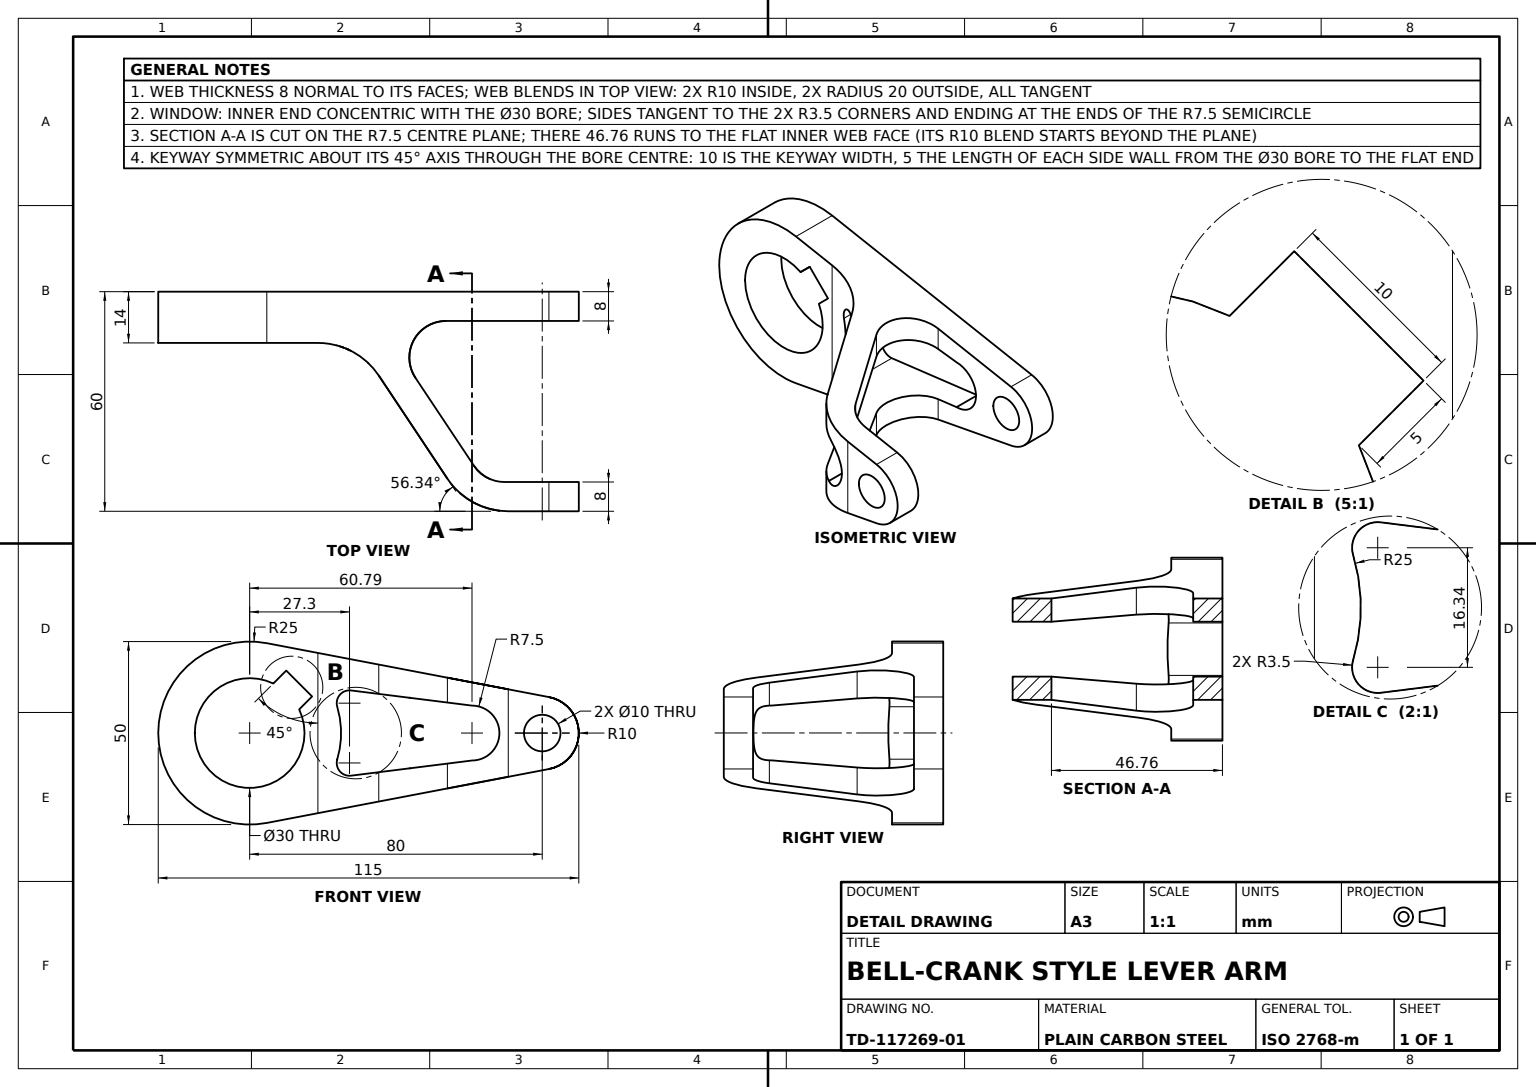
from build123d import *

# Parameters (mm, degrees)
LEVER_ARM_PROFILE_SKETCH_R = 5
LEVER_ARM_BODY_DEPTH       = 60
ARM_RELIEF_CUT_DEPTH       = 112.018016556
ARM_RELIEF_CUT_DEPTH_BACK  = 112.018016556


with BuildPart() as part:
    # Lever Arm Profile Sketch → Lever Arm Body (new body)
    with BuildSketch(Plane.XY):
        with BuildLine():
            Line((81.822654266, 9.832493652), (4.687544359, 24.556606604))
            ThreePointArc((4.687544359, 24.556606604), (-25, 0), (4.687544359, -24.556606604))
            Line((4.687544359, -24.556606604), (81.822654266, -9.832493652))
            ThreePointArc((81.822654266, -9.832493652), (90, 0), (81.822654266, 9.832493652))
        make_face()
        with Locations(Location((80, 0, 0), (0, 0, 180))):
            Circle(LEVER_ARM_PROFILE_SKETCH_R, mode=Mode.SUBTRACT)
        with BuildLine():
            Line((60.79258109, 7.5), (27.739398554, 11.641553498))
            ThreePointArc((27.739398554, 11.641553498), (24.632664937, 10.429819806), (23.951098456, 7.165534365))
            ThreePointArc((23.951098456, 7.165534365), (25, 0), (23.951098456, -7.165534365))
            ThreePointArc((23.951098456, -7.165534365), (24.632664937, -10.429819806), (27.739398554, -11.641553498))
            Line((27.739398554, -11.641553498), (60.79258109, -7.5))
            ThreePointArc((60.79258109, -7.5), (68.29258109, 0), (60.79258109, 7.5))
        make_face(mode=Mode.SUBTRACT)
        with BuildLine():
            Line((10, 17.071067812), (6.464466094, 13.535533906))
            ThreePointArc((6.464466094, 13.535533906), (-10.606601718, -10.606601718), (13.535533906, 6.464466094))
            Line((13.535533906, 6.464466094), (17.071067812, 10))
            Line((17.071067812, 10), (10, 17.071067812))
        make_face(mode=Mode.SUBTRACT)
    extrude(amount=LEVER_ARM_BODY_DEPTH)

    # Relief Cut Profile Sketch → Arm Relief Cut (cut, two sides: drawn at the far end of the back side and taken through both)
    with BuildSketch(Plane(origin=(0, 0, 0), x_dir=(1, 0, 0), z_dir=(0, 1, 0)).offset(-ARM_RELIEF_CUT_DEPTH_BACK)):
        with BuildLine():
            Line((18.654539923, -14), (-25, -14))
            Line((-25, -14), (-25, -60))
            Line((-25, -60), (70.709652312, -60))
            ThreePointArc((70.709652312, -60), (61.268398012, -57.631299364), (54.063494219, -51.086271725))
            Line((54.063494219, -51.086271725), (35.300698016, -22.913728275))
            ThreePointArc((35.300698016, -22.913728275), (28.095794223, -16.368700636), (18.654539923, -14))
        make_face()
        with BuildLine():
            Line((53.654787377, -8), (90, -8))
            Line((90, -8), (90, -52))
            Line((90, -52), (69.638687081, -52))
            ThreePointArc((69.638687081, -52), (64.918059931, -50.815649682), (61.315608035, -47.543135862))
            Line((61.315608035, -47.543135862), (45.331708331, -23.543135862))
            ThreePointArc((45.331708331, -23.543135862), (44.839137696, -13.27937285), (53.654787377, -8))
        make_face()
    extrude(amount=ARM_RELIEF_CUT_DEPTH + ARM_RELIEF_CUT_DEPTH_BACK, mode=Mode.SUBTRACT)


solid = part.part
